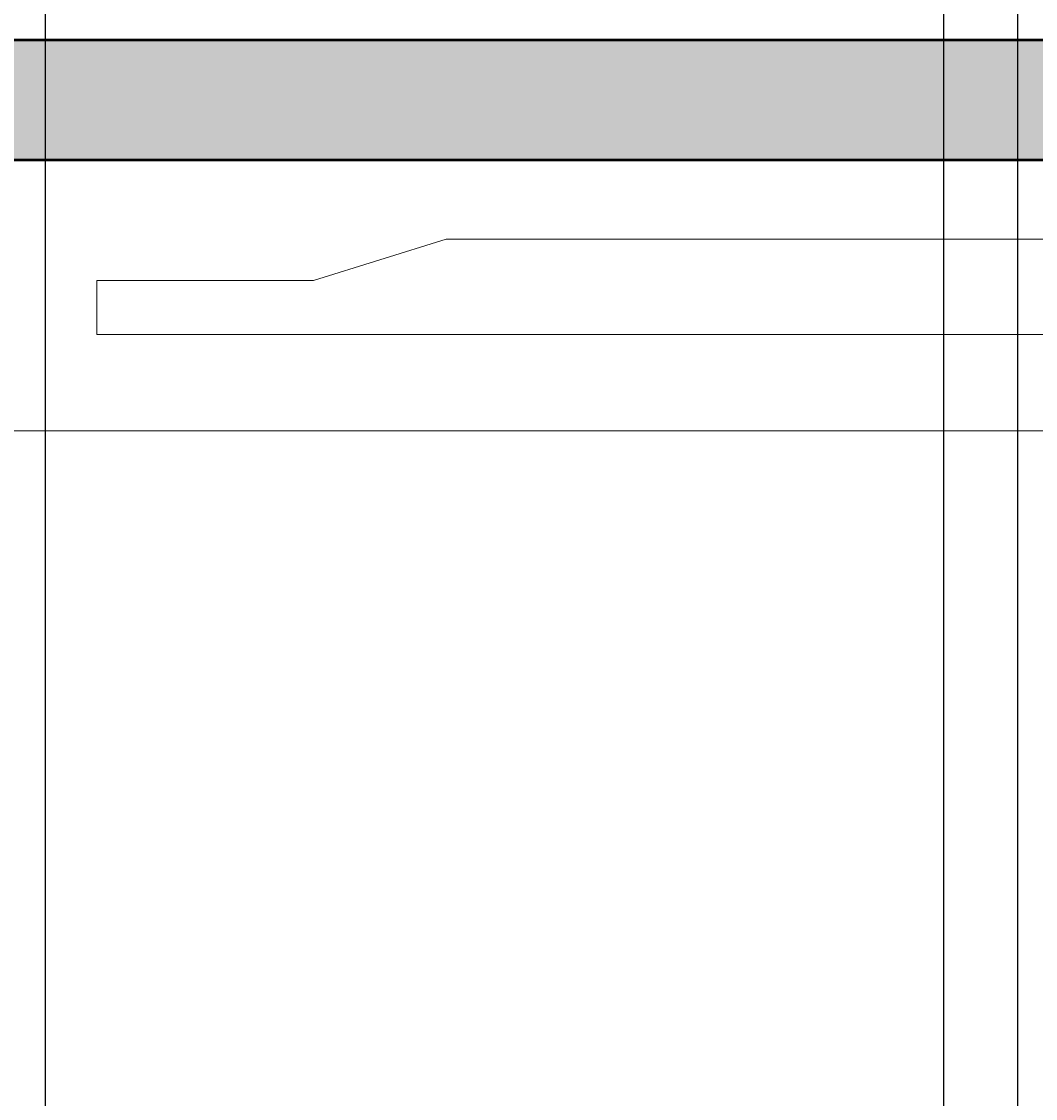
# Model space of a CAD drawing. Units: inches. Extents: x 2231 to 2461, y 2045 to 2455.
# Tile 51 of 95: x 2262 to 2295, y 2271 to 2307. Entities that reach past the tile are written whole.
import ezdxf

# ---------------------------------------------------------------- set-up
doc = ezdxf.new("R2010")
doc.units = ezdxf.units.IN
for name, color, linetype, lineweight in [('A-ANNO-DIMS', 2, 'Continuous', 18), ('A-EQPM', 8, 'Continuous', 18), ('A-FURN', 9, 'Continuous', 18), ('A-WALL', 7, 'Continuous', 50)]:
    doc.layers.add(name, color=color, linetype=linetype, lineweight=lineweight)
doc.layers.add('A-WALL-PATT', color=18, linetype='Continuous', lineweight=13, true_color=0x000000)
doc.styles.get("Standard").update_dxf_attribs({"font": 'arial.ttf'})
doc.dimstyles.get("Standard").update_dxf_attribs({"dimtxt": 0.18, "dimasz": 0.18, "dimexe": 0.18, "dimexo": 0.0625, "dimgap": 0.09, "dimtad": 0, "dimtih": 1, "dimtoh": 1, "dimdec": 4, "dimzin": 0, "dimdsep": 46, "dimtxsty": 'Standard', "dimcen": 0.09, "dimadec": 0, "dimazin": 0, "dimtfac": 1, "dimtdec": 4, "dimtofl": 0, "dimtmove": 0, "dimatfit": 3, "dimfxl": 1, "dimtolj": 1, "dimtzin": 0, "dimarcsym": 0})

# ---------------------------------------------------------------- blocks, each defined once
blk = doc.blocks.new('*D47')
at = {"layer": 'A-ANNO-DIMS', "color": 0, "lineweight": -2, "transparency": 16777216}
for p, q in [((2258.794, 2182.895), (2258.794, 2454.645)), ((2258.974, 2454.465), (2276.575, 2454.465)), ((2294.614, 2454.465), (2277.012, 2454.465)), ((2294.794, 2182.895), (2294.794, 2454.645))]:
    blk.add_line(p, q, dxfattribs=at)
at = {"layer": 'A-ANNO-DIMS', "color": 0, "transparency": 16777216}
for points in [[(2258.974, 2454.495), (2258.974, 2454.435), (2258.794, 2454.465)], [(2294.614, 2454.495), (2294.614, 2454.435), (2294.794, 2454.465)]]:
    blk.add_solid(points, dxfattribs=at)
at = {"layer": 'Defpoints', "color": 0, "transparency": 16777216}
for p in [(2294.794, 2454.465), (2258.794, 2182.833), (2294.794, 2182.833)]:
    blk.add_point(p, dxfattribs=at)
at = {"layer": 'A-ANNO-DIMS', "color": 0, "transparency": 16777216, "insert": (2276.794, 2454.465), "char_height": 0.18, "attachment_point": 5}
blk.add_mtext('\\A1;36', dxfattribs=at)
blk = doc.blocks.new('*D51')
at = {"layer": 'A-ANNO-DIMS', "color": 0, "lineweight": -2, "transparency": 16777216}
for p, q in [((2258.794, 2306.77), (2258.794, 2044.803)), ((2330.794, 2306.77), (2330.794, 2044.803)), ((2258.974, 2044.983), (2294.576, 2044.983)), ((2330.614, 2044.983), (2295.011, 2044.983))]:
    blk.add_line(p, q, dxfattribs=at)
at = {"layer": 'A-ANNO-DIMS', "color": 0, "transparency": 16777216}
for points in [[(2258.974, 2045.013), (2258.974, 2044.953), (2258.794, 2044.983)], [(2330.614, 2045.013), (2330.614, 2044.953), (2330.794, 2044.983)]]:
    blk.add_solid(points, dxfattribs=at)
at = {"layer": 'Defpoints', "color": 0, "transparency": 16777216}
for p in [(2258.794, 2306.833), (2330.794, 2306.833), (2330.794, 2044.983)]:
    blk.add_point(p, dxfattribs=at)
at = {"layer": 'A-ANNO-DIMS', "color": 0, "transparency": 16777216, "insert": (2294.794, 2044.983), "char_height": 0.18, "attachment_point": 5}
blk.add_mtext('\\A1;72', dxfattribs=at)
blk = doc.blocks.new('*D62')
at = {"layer": 'A-ANNO-DIMS', "color": 0, "lineweight": -2, "transparency": 16777216}
for p, q in [((2262.321, 2255.176), (2262.321, 2454.645)), ((2262.501, 2454.465), (2277.102, 2454.465)), ((2292.141, 2454.465), (2277.539, 2454.465)), ((2292.321, 2253.176), (2292.321, 2454.645))]:
    blk.add_line(p, q, dxfattribs=at)
at = {"layer": 'A-ANNO-DIMS', "color": 0, "transparency": 16777216}
for points in [[(2262.501, 2454.495), (2262.501, 2454.435), (2262.321, 2454.465)], [(2292.141, 2454.495), (2292.141, 2454.435), (2292.321, 2454.465)]]:
    blk.add_solid(points, dxfattribs=at)
at = {"layer": 'Defpoints', "color": 0, "transparency": 16777216}
for p in [(2292.321, 2454.465), (2262.321, 2255.114), (2292.321, 2253.114)]:
    blk.add_point(p, dxfattribs=at)
at = {"layer": 'A-ANNO-DIMS', "color": 0, "transparency": 16777216, "insert": (2277.321, 2454.465), "char_height": 0.18, "attachment_point": 5}
blk.add_mtext('\\A1;30', dxfattribs=at)

msp = doc.modelspace()

# ---------------------------------------------------------------- hatches: boundary and pattern name
at = {"layer": 'A-WALL-PATT'}
h = msp.add_hatch(color=256, dxfattribs=at)
h.dxf.hatch_style = 1
h.paths.add_polyline_path([(2441.7935, 2269.1535), (2432.7935, 2269.1535), (2432.7935, 2186.8328), (2396.7935, 2186.8328), (2396.7935, 2286.8328), (2394.7935, 2286.8328), (2394.7935, 2186.8328), (2334.7935, 2186.8328), (2334.7935, 2182.8328), (2432.7935, 2182.8328), (2432.7935, 2072.8328), (2416.6639, 2072.8328), (2416.6639, 2063.8328), (2441.7935, 2063.8328)])
h.paths.add_polyline_path([(2368.6639, 2072.8328), (2367.04, 2072.8328), (2330.7942, 2072.8328), (2330.7397, 2063.8328), (2368.6639, 2063.8328)])
h.paths.add_polyline_path([(2300.7392, 2068.3328), (2300.7392, 2072.8328), (2298.7935, 2072.8328), (2294.7935, 2072.8328), (2258.7935, 2072.8328), (2258.7935, 2120.8328), (2294.7935, 2120.8328), (2298.7935, 2120.8328), (2298.7935, 2128.8328), (2294.7935, 2128.8328), (2294.7935, 2124.8328), (2258.7935, 2124.8328), (2258.7935, 2182.8328), (2294.7935, 2182.8328), (2294.7935, 2174.8328), (2298.7935, 2174.8328), (2298.7935, 2182.8328), (2304.7935, 2182.8328), (2304.7935, 2186.8328), (2258.7935, 2186.8328), (2258.7935, 2221.999), (2249.7935, 2221.999), (2249.7935, 2063.8328), (2300.7392, 2063.8328)])
h.paths.add_polyline_path([(2391.9338, 2435.8328), (2333.82, 2435.8328), (2333.82, 2426.8328), (2368.7935, 2426.8328), (2368.7935, 2374.9508), (2368.7935, 2370.8328), (2372.3935, 2370.8328), (2372.7935, 2370.8328), (2372.7935, 2426.8328), (2391.9338, 2426.8328)])
h.paths.add_polyline_path([(2441.7935, 2435.8328), (2415.9338, 2435.8328), (2415.9338, 2426.8328), (2432.7935, 2426.8328), (2432.7935, 2334.8328), (2372.7935, 2334.8328), (2372.7935, 2346.8328), (2368.7935, 2346.8328), (2368.7935, 2306.8328), (2360.7935, 2306.8328), (2360.7935, 2302.8328), (2368.7935, 2302.8328), (2372.7935, 2302.8328), (2372.7935, 2330.8328), (2432.7935, 2330.8328), (2432.7935, 2317.1535), (2441.7935, 2317.1535)])
h.paths.add_polyline_path([(2285.82, 2435.8328), (2249.7935, 2435.8328), (2249.7935, 2269.999), (2258.7935, 2269.999), (2258.7935, 2302.8328), (2318.8168, 2302.8328), (2330.7935, 2302.8328), (2330.7935, 2306.8328), (2258.7935, 2306.8328), (2258.7935, 2426.8328), (2285.82, 2426.8328)])

# ---------------------------------------------------------------- linework, layer by layer
at = {"layer": 'A-EQPM'}
msp.add_line((2275.7007, 2300.1814), (2271.2638, 2298.7991), dxfattribs=at)
for points in [[(2275.7007, 2300.1814), (2300.1765, 2300.1814)], [(2304.5787, 2298.7991), (2311.8486, 2298.7991), (2311.8486, 2296.9979), (2264.0286, 2296.9979), (2264.0286, 2298.7991), (2271.2638, 2298.7991)]]:
    msp.add_lwpolyline(points, dxfattribs=at)
at = {"layer": 'A-FURN'}
msp.add_lwpolyline([(2258.7935, 2302.8328), (2318.8168, 2302.8328), (2318.8168, 2293.7759), (2258.7935, 2293.7759)], close=True, dxfattribs=at)
at = {"layer": 'A-WALL'}
for p, q in [((2258.7935, 2306.8328), (2330.7935, 2306.8328)), ((2258.7935, 2302.8328), (2330.7935, 2302.8328))]:
    msp.add_line(p, q, dxfattribs=at)

# ---------------------------------------------------------------- dimensions: what is measured, and where the dimension line sits
at = {"layer": 'A-ANNO-DIMS'}
for base, p1, p2, picture, middle in [((2294.7935, 2454.4653), (2258.7935, 2182.8328), (2294.7935, 2182.8328), '*D47', (2276.7935, 2454.4653)), ((2292.3207, 2454.4653), (2262.3207, 2255.1137), (2292.3207, 2253.1137), '*D62', (2277.3207, 2454.4653)), ((2330.7935, 2044.9825), (2258.7935, 2306.8328), (2330.7935, 2306.8328), '*D51', (2294.7935, 2044.9825))]:
    dim = msp.add_linear_dim(base=base, p1=p1, p2=p2, dimstyle='Standard', override={"dimdec": 0, "dimlfac": 1, "dimrnd": 0, "dimzin": 0, "dimdsep": 46, "dimlunit": 2}, dxfattribs=at)
    dim.commit()
    dim.dimension.update_dxf_attribs({"geometry": picture, "text_midpoint": middle})

doc.saveas('drawing.dxf')
